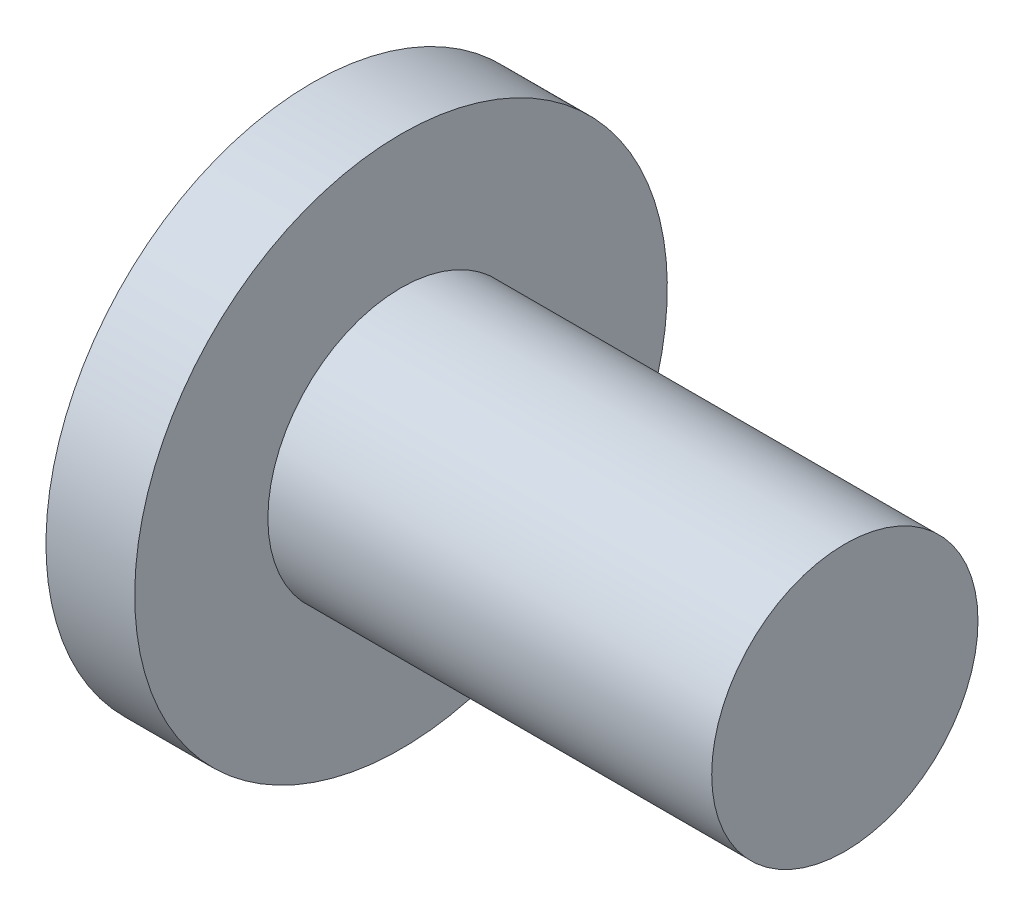
ISO-10303-21;
HEADER;
FILE_DESCRIPTION(('STEP AP214'),'2;1');
FILE_NAME('part.step','',(''),(''),'','','');
FILE_SCHEMA(('AUTOMOTIVE_DESIGN { 1 0 10303 214 1 1 1 1 }'));
ENDSEC;
DATA;
#1=APPLICATION_CONTEXT('core data for automotive mechanical design processes');
#2=APPLICATION_PROTOCOL_DEFINITION('international standard','automotive_design',2000,#1);
#3=PRODUCT_CONTEXT('',#1,'mechanical');
#4=PRODUCT('Part','Part','',(#3));
#5=PRODUCT_RELATED_PRODUCT_CATEGORY('part','',(#4));
#6=PRODUCT_DEFINITION_FORMATION('','',#4);
#7=PRODUCT_DEFINITION_CONTEXT('part definition',#1,'design');
#8=PRODUCT_DEFINITION('design','',#6,#7);
#9=PRODUCT_DEFINITION_SHAPE('','',#8);
#10=(LENGTH_UNIT() NAMED_UNIT(*) SI_UNIT(.MILLI.,.METRE.));
#11=(NAMED_UNIT(*) PLANE_ANGLE_UNIT() SI_UNIT($,.RADIAN.));
#12=(NAMED_UNIT(*) SI_UNIT($,.STERADIAN.) SOLID_ANGLE_UNIT());
#13=UNCERTAINTY_MEASURE_WITH_UNIT(LENGTH_MEASURE(1.E-05),#10,'distance_accuracy_value','');
#14=(GEOMETRIC_REPRESENTATION_CONTEXT(3) GLOBAL_UNCERTAINTY_ASSIGNED_CONTEXT((#13)) GLOBAL_UNIT_ASSIGNED_CONTEXT((#10,
#11,#12)) REPRESENTATION_CONTEXT('',''));
#15=CARTESIAN_POINT('',(0.,0.,0.));
#16=DIRECTION('',(0.,0.,1.));
#17=DIRECTION('',(1.,0.,0.));
#18=AXIS2_PLACEMENT_3D('',#15,#16,#17);
#19=CARTESIAN_POINT('',(0.,3.,0.));
#20=DIRECTION('',(1.,0.,0.));
#21=DIRECTION('',(0.,1.,0.));
#22=AXIS2_PLACEMENT_3D('',#19,#20,#21);
#23=PLANE('',#22);
#24=CARTESIAN_POINT('',(0.,0.,0.));
#25=DIRECTION('',(1.,0.,0.));
#26=DIRECTION('',(0.,1.,0.));
#27=AXIS2_PLACEMENT_3D('',#24,#25,#26);
#28=CIRCLE('',#27,3.);
#29=CARTESIAN_POINT('',(0.,3.,0.));
#30=VERTEX_POINT('',#29);
#31=EDGE_CURVE('E51',#30,#30,#28,.T.);
#32=ORIENTED_EDGE('',*,*,#31,.T.);
#33=EDGE_LOOP('',(#32));
#34=FACE_BOUND('',#33,.T.);
#35=ADVANCED_FACE('F40',(#34),#23,.T.);
#36=CARTESIAN_POINT('',(-12.,0.,0.));
#37=DIRECTION('',(-1.,0.,0.));
#38=DIRECTION('',(0.,-1.,0.));
#39=AXIS2_PLACEMENT_3D('',#36,#37,#38);
#40=PLANE('',#39);
#41=CARTESIAN_POINT('',(-12.,0.,0.));
#42=DIRECTION('',(1.,0.,0.));
#43=DIRECTION('',(0.,1.,0.));
#44=AXIS2_PLACEMENT_3D('',#41,#42,#43);
#45=CIRCLE('',#44,6.);
#46=CARTESIAN_POINT('',(-12.,6.,0.));
#47=VERTEX_POINT('',#46);
#48=EDGE_CURVE('E10',#47,#47,#45,.T.);
#49=ORIENTED_EDGE('',*,*,#48,.F.);
#50=EDGE_LOOP('',(#49));
#51=FACE_BOUND('',#50,.T.);
#52=ADVANCED_FACE('F66',(#51),#40,.T.);
#53=CARTESIAN_POINT('',(0.,0.,0.));
#54=DIRECTION('',(1.,0.,0.));
#55=DIRECTION('',(0.,1.,0.));
#56=AXIS2_PLACEMENT_3D('',#53,#54,#55);
#57=CYLINDRICAL_SURFACE('',#56,6.);
#58=ORIENTED_EDGE('',*,*,#48,.T.);
#59=EDGE_LOOP('',(#58));
#60=FACE_BOUND('',#59,.T.);
#61=CARTESIAN_POINT('',(-10.,0.,0.));
#62=DIRECTION('',(1.,0.,0.));
#63=DIRECTION('',(0.,1.,0.));
#64=AXIS2_PLACEMENT_3D('',#61,#62,#63);
#65=CIRCLE('',#64,6.);
#66=CARTESIAN_POINT('',(-10.,6.,0.));
#67=VERTEX_POINT('',#66);
#68=EDGE_CURVE('E43',#67,#67,#65,.T.);
#69=ORIENTED_EDGE('',*,*,#68,.F.);
#70=EDGE_LOOP('',(#69));
#71=FACE_BOUND('',#70,.T.);
#72=ADVANCED_FACE('F67',(#60,#71),#57,.T.);
#73=CARTESIAN_POINT('',(-10.,6.,0.));
#74=DIRECTION('',(1.,0.,0.));
#75=DIRECTION('',(0.,1.,0.));
#76=AXIS2_PLACEMENT_3D('',#73,#74,#75);
#77=PLANE('',#76);
#78=ORIENTED_EDGE('',*,*,#68,.T.);
#79=EDGE_LOOP('',(#78));
#80=FACE_BOUND('',#79,.T.);
#81=CARTESIAN_POINT('',(-10.,0.,0.));
#82=DIRECTION('',(1.,0.,0.));
#83=DIRECTION('',(0.,1.,0.));
#84=AXIS2_PLACEMENT_3D('',#81,#82,#83);
#85=CIRCLE('',#84,3.);
#86=CARTESIAN_POINT('',(-10.,3.,0.));
#87=VERTEX_POINT('',#86);
#88=EDGE_CURVE('E50',#87,#87,#85,.T.);
#89=ORIENTED_EDGE('',*,*,#88,.F.);
#90=EDGE_LOOP('',(#89));
#91=FACE_BOUND('',#90,.T.);
#92=ADVANCED_FACE('F58',(#80,#91),#77,.T.);
#93=CARTESIAN_POINT('',(0.,0.,0.));
#94=DIRECTION('',(1.,0.,0.));
#95=DIRECTION('',(0.,1.,0.));
#96=AXIS2_PLACEMENT_3D('',#93,#94,#95);
#97=CYLINDRICAL_SURFACE('',#96,3.);
#98=ORIENTED_EDGE('',*,*,#88,.T.);
#99=EDGE_LOOP('',(#98));
#100=FACE_BOUND('',#99,.T.);
#101=ORIENTED_EDGE('',*,*,#31,.F.);
#102=EDGE_LOOP('',(#101));
#103=FACE_BOUND('',#102,.T.);
#104=ADVANCED_FACE('F59',(#100,#103),#97,.T.);
#105=CLOSED_SHELL('',(#35,#52,#72,#92,#104));
#106=MANIFOLD_SOLID_BREP('B2',#105);
#107=ADVANCED_BREP_SHAPE_REPRESENTATION('',(#18,#106),#14);
#108=SHAPE_DEFINITION_REPRESENTATION(#9,#107);
ENDSEC;
END-ISO-10303-21;
